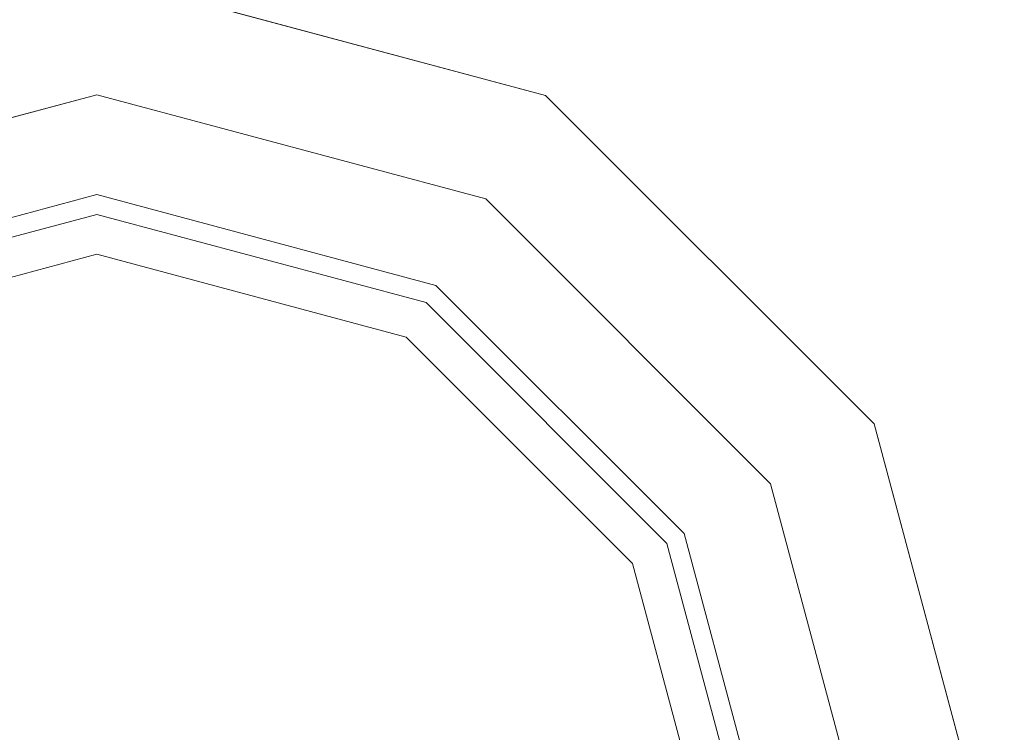
# Model space of a CAD drawing. Units: inches. Extents: x 375 to 1122, y 27 to 1069.
# Tile 88 of 155: x 725.203 to 731.282, y 854.634 to 859.033. Entities that reach past the tile are written whole.
import ezdxf

# ---------------------------------------------------------------- set-up
doc = ezdxf.new("R2010")
doc.units = ezdxf.units.IN
doc.layers.add('A-ANNO-DIMS', color=2, linetype='Continuous', lineweight=18)
doc.layers.add('Furniture', color=30, linetype='Continuous', lineweight=18)
doc.styles.get("Standard").update_dxf_attribs({"font": 'arial.ttf'})
doc.dimstyles.new('ISO-25', dxfattribs={"dimtxt": 12, "dimasz": 2.5, "dimexe": 1.5, "dimexo": 1.5, "dimtad": 1, "dimdec": 1, "dimlunit": 3, "dimtxsty": 'Standard', "dimblk": 'ARCHTICK', "dimcen": 2.5, "dimadec": 0, "dimazin": 0, "dimtfac": 1, "dimtdec": 1, "dimtmove": 0, "dimatfit": 3, "dimfxl": 1.5, "dimfxlon": 1, "dimarcsym": 0})

# ---------------------------------------------------------------- blocks, each defined once
blk = doc.blocks.new('A$C403C54AD')
at = {"linetype": 'ByBlock', "invisible_edges": 5}
for points in [[(2.11411, 1.15687, -0.03783), (2.11411, 1.1384, -0.03783), (2.05409, 1.12232, -0.03783), (2.04485, 1.13831, -0.03783)], [(2.11411, 1.12301, -0.05168), (2.11411, 1.15687, -0.04244), (2.04485, 1.13831, -0.04244), (2.06178, 1.10899, -0.05168)], [(2.04485, 1.13831, -0.03783), (2.05409, 1.12232, -0.03783), (2.01014, 1.07837, -0.03783), (1.99415, 1.08761, -0.03783)], [(2.06178, 1.10899, -0.05168), (2.04485, 1.13831, -0.04244), (1.99415, 1.08761, -0.04244), (2.02347, 1.07068, -0.05168)], [(2.11411, 1.1384, -0.03783), (2.11411, 1.11993, -0.04398), (2.06332, 1.10632, -0.04398), (2.05409, 1.12232, -0.03783)], [(2.05409, 1.12232, -0.03783), (2.06332, 1.10632, -0.04398), (2.02614, 1.06914, -0.04398), (2.01014, 1.07837, -0.03783)], [(2.11411, 1.11377, -0.06091), (2.11411, 1.12301, -0.05168), (2.06178, 1.10899, -0.05168), (2.0664, 1.10099, -0.06091)], [(2.11411, 1.11993, -0.04398), (2.11411, 1.01834, -0.04398), (2.11411, 1.01834, -0.04398), (2.06332, 1.10632, -0.04398)], [(2.0664, 1.10099, -0.06091), (2.06178, 1.10899, -0.05168), (2.02347, 1.07068, -0.05168), (2.03147, 1.06606, -0.06091)], [(2.06332, 1.10632, -0.04398), (2.11411, 1.01834, -0.04398), (2.11411, 1.01834, -0.04398), (2.02614, 1.06914, -0.04398)], [(1.99415, 1.08761, -0.03783), (2.01014, 1.07837, -0.03783), (1.99406, 1.01834, -0.03783), (1.97559, 1.01834, -0.03783)], [(2.02347, 1.07068, -0.05168), (1.99415, 1.08761, -0.04244), (1.97559, 1.01834, -0.04244), (2.00945, 1.01834, -0.05168)], [(2.01014, 1.07837, -0.03783), (2.02614, 1.06914, -0.04398), (2.01253, 1.01834, -0.04398), (1.99406, 1.01834, -0.03783)], [(2.03147, 1.06606, -0.06091), (2.02347, 1.07068, -0.05168), (2.00945, 1.01834, -0.05168), (2.01868, 1.01834, -0.06091)], [(2.02614, 1.06914, -0.04398), (2.11411, 1.01834, -0.04398), (2.11411, 1.01834, -0.04398), (2.01253, 1.01834, -0.04398)], [(1.97559, 1.01834, -0.03783), (1.99406, 1.01834, -0.03783), (2.01014, 0.95832, -0.03783), (1.99415, 0.94908, -0.03783)], [(2.00945, 1.01834, -0.05168), (1.97559, 1.01834, -0.04244), (1.99415, 0.94908, -0.04244), (2.02347, 0.96601, -0.05168)], [(1.99406, 1.01834, -0.03783), (2.01253, 1.01834, -0.04398), (2.02614, 0.96755, -0.04398), (2.01014, 0.95832, -0.03783)], [(2.01868, 1.01834, -0.06091), (2.00945, 1.01834, -0.05168), (2.02347, 0.96601, -0.05168), (2.03147, 0.97063, -0.06091)], [(2.01253, 1.01834, -0.04398), (2.11411, 1.01834, -0.04398), (2.11411, 1.01834, -0.04398), (2.02614, 0.96755, -0.04398)], [(2.02614, 0.96755, -0.04398), (2.11411, 1.01834, -0.04398), (2.11411, 1.01834, -0.04398), (2.06332, 0.93037, -0.04398)], [(2.06332, 0.93037, -0.04398), (2.11411, 1.01834, -0.04398), (2.11411, 1.01834, -0.04398), (2.11411, 0.91676, -0.04398)]]:
    blk.add_3dface(points, dxfattribs=at)
at = {"linetype": 'ByBlock'}
for points in [[(2.11411, 1.15687, -0.04244), (2.11411, 1.15687, -0.03783), (2.04485, 1.13831, -0.03783), (2.04485, 1.13831, -0.04244)], [(2.04485, 1.13831, -0.04244), (2.04485, 1.13831, -0.03783), (1.99415, 1.08761, -0.03783), (1.99415, 1.08761, -0.04244)], [(1.99415, 1.08761, -0.04244), (1.99415, 1.08761, -0.03783), (1.97559, 1.01834, -0.03783), (1.97559, 1.01834, -0.04244)], [(1.97559, 1.01834, -0.04244), (1.97559, 1.01834, -0.03783), (1.99415, 0.94908, -0.03783), (1.99415, 0.94908, -0.04244)]]:
    blk.add_3dface(points, dxfattribs=at)
blk = doc.blocks.new('_ArchTick')
at = {"color": 0, "linetype": 'ByBlock', "const_width": 0.15}
blk.add_lwpolyline([(-0.5, -0.5), (0.5, 0.5)], dxfattribs=at)
blk = doc.blocks.new('*D85')
at = {"layer": 'A-ANNO-DIMS', "color": 0, "lineweight": -2, "transparency": 16777216}
for p, q in [((401.5073, 868.5277), (398.5073, 868.5277)), ((400.0073, 814.5277), (400.0073, 868.5277)), ((401.5073, 814.5277), (398.5073, 814.5277))]:
    blk.add_line(p, q, dxfattribs=at)
at = {"layer": 'Defpoints', "color": 0, "transparency": 16777216}
for p in [(400.0073, 868.5277), (845.0073, 868.5277), (845.0073, 814.5277)]:
    blk.add_point(p, dxfattribs=at)
at = {"layer": 'A-ANNO-DIMS', "color": 0, "lineweight": -2, "transparency": 16777216, "xscale": 2.5, "yscale": 2.5, "zscale": 2.5}
for p, rotation in [((400.0073, 868.5277), 90), ((400.0073, 814.5277), 270)]:
    blk.add_blockref('_ArchTick', p, dxfattribs=dict(at, rotation=rotation))
at = {"layer": 'A-ANNO-DIMS', "color": 0, "transparency": 16777216, "insert": (393.2555, 841.5277), "char_height": 12, "attachment_point": 5, "rotation": 90}
blk.add_mtext('4\'-6"', dxfattribs=at)
blk = doc.blocks.new('*D88')
at = {"layer": 'A-ANNO-DIMS', "color": 0, "lineweight": -2, "transparency": 16777216}
for p, q in [((731.0073, 1052.5277), (731.0073, 1055.5277)), ((854.0073, 1052.5277), (854.0073, 1055.5277)), ((731.0073, 1054.0277), (854.0073, 1054.0277))]:
    blk.add_line(p, q, dxfattribs=at)
at = {"layer": 'Defpoints', "color": 0, "transparency": 16777216}
for p in [(854.0073, 1054.0277), (731.0073, 502.5277), (854.0073, 502.5277)]:
    blk.add_point(p, dxfattribs=at)
at = {"layer": 'A-ANNO-DIMS', "color": 0, "lineweight": -2, "transparency": 16777216, "xscale": 2.5, "yscale": 2.5, "zscale": 2.5, "rotation": 180}
blk.add_blockref('_ArchTick', (731.0073, 1054.0277), dxfattribs=at)
at = {"layer": 'A-ANNO-DIMS', "color": 0, "lineweight": -2, "transparency": 16777216, "xscale": 2.5, "yscale": 2.5, "zscale": 2.5}
blk.add_blockref('_ArchTick', (854.0073, 1054.0277), dxfattribs=at)
at = {"layer": 'A-ANNO-DIMS', "color": 0, "transparency": 16777216, "insert": (792.5073, 1060.7837), "char_height": 12, "attachment_point": 5}
blk.add_mtext('10\'-3"', dxfattribs=at)
blk = doc.blocks.new('*D91')
at = {"layer": 'A-ANNO-DIMS', "color": 0, "lineweight": -2, "transparency": 16777216}
for p, q in [((728.0073, 1052.5277), (728.0073, 1055.5277)), ((788.0073, 1052.5277), (788.0073, 1055.5277)), ((728.0073, 1054.0277), (788.0073, 1054.0277))]:
    blk.add_line(p, q, dxfattribs=at)
at = {"layer": 'Defpoints', "color": 0, "transparency": 16777216}
for p in [(788.0073, 1054.0277), (728.0073, 774.0277), (788.0073, 774.0277)]:
    blk.add_point(p, dxfattribs=at)
at = {"layer": 'A-ANNO-DIMS', "color": 0, "lineweight": -2, "transparency": 16777216, "xscale": 2.5, "yscale": 2.5, "zscale": 2.5, "rotation": 180}
blk.add_blockref('_ArchTick', (728.0073, 1054.0277), dxfattribs=at)
at = {"layer": 'A-ANNO-DIMS', "color": 0, "lineweight": -2, "transparency": 16777216, "xscale": 2.5, "yscale": 2.5, "zscale": 2.5}
blk.add_blockref('_ArchTick', (788.0073, 1054.0277), dxfattribs=at)
at = {"layer": 'A-ANNO-DIMS', "color": 0, "transparency": 16777216, "insert": (758.0073, 1060.7796), "char_height": 12, "attachment_point": 5}
blk.add_mtext('5\'-0"', dxfattribs=at)

msp = doc.modelspace()

# ---------------------------------------------------------------- block references
at = {"layer": 'Furniture', "xscale": 39.9918517141215, "yscale": 39.9918517141215, "zscale": 39.9918517141215, "rotation": 270}
msp.add_blockref('A$C403C54AD', (684.9549, 938.3156, 0.024), dxfattribs=at)

# ---------------------------------------------------------------- dimensions: what is measured, and where the dimension line sits
at = {"layer": 'A-ANNO-DIMS'}
for base, p1, p2, picture, middle in [((788.0073, 1054.0277), (728.0073, 774.0277), (788.0073, 774.0277), '*D91', (758.0073, 1060.7796)), ((854.0073, 1054.0277), (731.0073, 502.5277), (854.0073, 502.5277), '*D88', (792.5073, 1060.7837))]:
    dim = msp.add_linear_dim(base=base, p1=p1, p2=p2, dimstyle='ISO-25', override={"dimdec": 1, "dimlfac": 1, "dimrnd": 0, "dimzin": 1, "dimdsep": 46, "dimlunit": 4, "dimfrac": 2}, dxfattribs=at)
    dim.commit()
    dim.dimension.update_dxf_attribs({"geometry": picture, "text_midpoint": middle})
dim = msp.add_linear_dim(base=(400.0073, 868.5277), p1=(845.0073, 814.5277), p2=(845.0073, 868.5277), angle=90, dimstyle='ISO-25', override={"dimdec": 1, "dimlfac": 1, "dimrnd": 0, "dimzin": 1, "dimdsep": 46, "dimlunit": 4, "dimfrac": 2}, dxfattribs=at)
dim.commit()
dim.dimension.update_dxf_attribs({"geometry": '*D85', "text_midpoint": (393.2555, 841.5277)})

doc.saveas('drawing.dxf')
